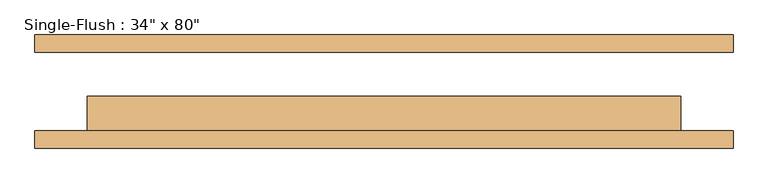
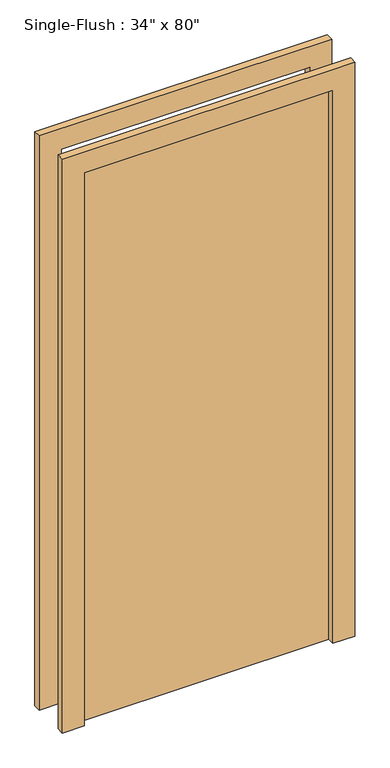
"""IFC4 building model written with IfcOpenShell, lengths in millimetres: door geometry."""

from ifc_helpers import new_model, si_unit, frame, origin, origin_with_axes, place, context, project, spatial, polyline, outline, extrude, source, transform, mapped, element, save


def door_825b8444(model_context):
    return source(origin(), model_context, "Body", "SweptSolid", [
        extrude(outline(polyline([(2108.2, -508.0), (0.0, -508.0), (0.0, -431.8), (2032.0, -431.8), (2032.0, 431.8), (0.0, 431.8), (0.0, 508.0), (2108.2, 508.0), (2108.2, -508.0)])), frame((0.0, -82.55, 0.0), z_axis=(0.0, 1.0, 0.0), x_axis=(0.0, 0.0, 1.0)), (0.0, 0.0, 1.0), 25.4),
        extrude(outline(polyline([(2108.2, 508.0), (2108.2, -508.0), (0.0, -508.0), (0.0, -431.8), (2032.0, -431.8), (2032.0, 431.8), (0.0, 431.8), (0.0, 508.0), (2108.2, 508.0)])), frame((0.0, 57.15, 0.0), z_axis=(0.0, 1.0, 0.0), x_axis=(0.0, 0.0, 1.0)), (0.0, 0.0, 1.0), 25.4),
        extrude(outline(polyline([(431.8, -6.35), (431.8, -57.15), (-431.8, -57.15), (-431.8, -6.35), (431.8, -6.35)])), origin_with_axes(), (0.0, 0.0, 1.0), 2032.0),
    ])


if __name__ == "__main__":
    model = new_model("IFC4")
    model_context = context("Model", 3, world=origin())
    ifc_project = project(units=[si_unit("LENGTHUNIT", "METRE", prefix="MILLI")], contexts=[model_context])
    site = spatial("IfcSite", under=ifc_project)
    building = spatial("IfcBuilding", under=site)
    placement = place(None, origin())
    door_shape = door_825b8444(model_context)
    element("IfcDoor", 1, ObjectType="Single-Flush : 34\" x 80\"", at=placement, inside=building, context=model_context, shape_type="MappedRepresentation", body=[
        mapped(door_shape, transform((0.0, 0.0, 0.0), x_axis=(1.0, 0.0, 0.0), y_axis=(0.0, 1.0, 0.0), z_axis=(0.0, 0.0, 1.0))),
    ])
    save(model, "model.ifc")

# Revit data of these elements
# Type "Single-Flush : 34\" x 80\""
#   Type Mark = "7"
#   Construction Type Id = "MDOOR"
#   Assembly Code = "C1020"
#   Analytic Construction = "Metal"
#   Thickness = 0' - 2"
#   Heat Transfer Coefficient (U) = 0.651978 BTU/(h·ft²·°F)
#   Height = 6' - 8"
#   Trim Projection Ext = 0' - 1"
#   Trim Projection Int = 0' - 1"
#   Trim Width = 0' - 3"
#   Width = 2' - 10"
#   Define Thermal Properties by = 1
#   Define Thermal Properties by = 1
#   Door Material = Door - Panel
#   Frame Material = Door - Frame
#   Visual Light Transmittance = 0
#   Solar Heat Gain Coefficient = 0
#   Function = (empty or 0)
#   Wall Closure = (empty or 0)
# Element 1 (IfcDoor, "Single-Flush : 34\" x 80\"")
#   Materials on its faces: "Door - Frame", "Door - Panel"
# Materials
#   "Door - Panel": class "Wood", colour RGB 210 159 95, transparency 0, Cost = 0
#   "Door - Frame": colour RGB 118 70 51, transparency 0, Cost = 0
